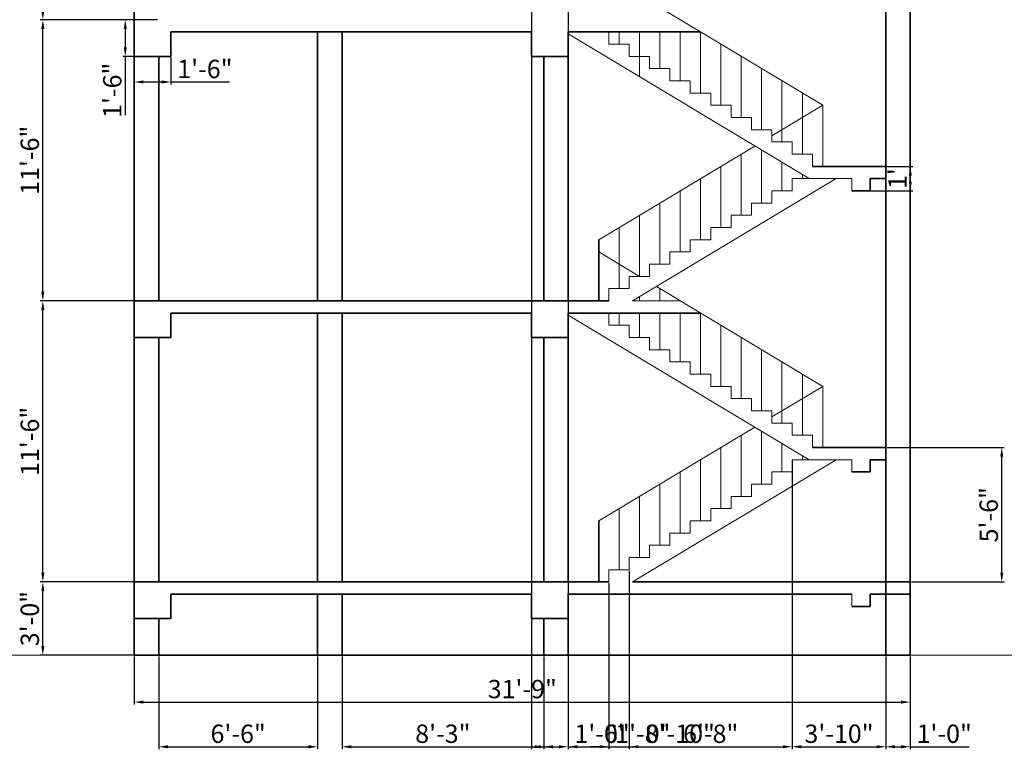
# Model space of a CAD drawing. Units: inches. Extents: x 1692 to 2762, y 798 to 1757.
# Tile 3 of 4: x 2279 to 2762, y 798 to 1156. Entities that reach past the tile are written whole.
import ezdxf

# ---------------------------------------------------------------- set-up
doc = ezdxf.new("R2010")
doc.units = ezdxf.units.IN
for name, color, linetype, lineweight in [('A-ANNO-DIMS', 2, 'Continuous', 18), ('A-CONS', 9, 'Continuous', 13), ('A-FLOR-STRS', 3, 'Continuous', 18), ('A-SECT', 1, 'Continuous', 35)]:
    doc.layers.add(name, color=color, linetype=linetype, lineweight=lineweight)
doc.styles.get("Standard").update_dxf_attribs({"font": 'arial.ttf'})
doc.dimstyles.new('ISO-25', dxfattribs={"dimtxt": 9, "dimasz": 4.5, "dimexe": 1.25, "dimexo": 0.625, "dimtad": 1, "dimdec": 0, "dimlunit": 3, "dimtxsty": 'Standard', "dimcen": 2.5, "dimadec": 0, "dimazin": 0, "dimtfac": 1, "dimtdec": 0, "dimtmove": 0, "dimatfit": 3, "dimfxl": 1, "dimarcsym": 0})

# ---------------------------------------------------------------- blocks, each defined once
blk = doc.blocks.new('*D4')
at = {"layer": 'A-ANNO-DIMS', "color": 0, "lineweight": -2, "transparency": 16777216}
for p, q in [((2334.78, 843.81), (2334.78, 820.21)), ((2715.78, 843.81), (2715.78, 820.21)), ((2339.28, 821.46), (2711.28, 821.46))]:
    blk.add_line(p, q, dxfattribs=at)
at = {"layer": 'A-ANNO-DIMS', "color": 0, "lineweight": 0, "transparency": 16777216}
for points in [[(2339.28, 822.21), (2339.28, 820.71), (2334.78, 821.46)], [(2711.28, 822.21), (2711.28, 820.71), (2715.78, 821.46)]]:
    blk.add_solid(points, dxfattribs=at)
at = {"layer": 'Defpoints', "color": 0, "lineweight": 0, "transparency": 16777216}
for p in [(2334.78, 844.43), (2715.78, 844.43), (2715.78, 821.46)]:
    blk.add_point(p, dxfattribs=at)
at = {"layer": 'A-ANNO-DIMS', "color": 0, "transparency": 16777216, "insert": (2525.28, 826.68), "char_height": 9, "attachment_point": 5}
blk.add_mtext('31\'-9"', dxfattribs=at)
blk = doc.blocks.new('*D5')
at = {"layer": 'A-ANNO-DIMS', "color": 0, "lineweight": -2, "transparency": 16777216}
for p, q in [((2346.16, 1156.43), (2329.11, 1156.43)), ((2330.36, 1151.93), (2330.36, 1142.93)), ((2346.16, 1138.43), (2329.11, 1138.43)), ((2330.36, 1138.43), (2330.36, 1109.61))]:
    blk.add_line(p, q, dxfattribs=at)
at = {"layer": 'A-ANNO-DIMS', "color": 0, "lineweight": 0, "transparency": 16777216}
for points in [[(2329.61, 1151.93), (2331.11, 1151.93), (2330.36, 1156.43)], [(2329.61, 1142.93), (2331.11, 1142.93), (2330.36, 1138.43)]]:
    blk.add_solid(points, dxfattribs=at)
at = {"layer": 'Defpoints', "color": 0, "lineweight": 0, "transparency": 16777216}
for p in [(2346.78, 1156.43), (2330.36, 1138.43), (2346.78, 1138.43)]:
    blk.add_point(p, dxfattribs=at)
at = {"layer": 'A-ANNO-DIMS', "color": 0, "transparency": 16777216, "insert": (2325.14, 1121.77), "char_height": 9, "attachment_point": 5, "rotation": 90}
blk.add_mtext('1\'-6"', dxfattribs=at)
blk = doc.blocks.new('*D6')
at = {"layer": 'A-ANNO-DIMS', "color": 0, "lineweight": -2, "transparency": 16777216}
for p, q in [((2334.78, 1137.81), (2334.78, 1124.62)), ((2352.78, 1137.81), (2352.78, 1124.62)), ((2339.28, 1125.87), (2348.28, 1125.87)), ((2352.78, 1125.87), (2381.61, 1125.87))]:
    blk.add_line(p, q, dxfattribs=at)
at = {"layer": 'A-ANNO-DIMS', "color": 0, "lineweight": 0, "transparency": 16777216}
for points in [[(2339.28, 1126.62), (2339.28, 1125.12), (2334.78, 1125.87)], [(2348.28, 1126.62), (2348.28, 1125.12), (2352.78, 1125.87)]]:
    blk.add_solid(points, dxfattribs=at)
at = {"layer": 'Defpoints', "color": 0, "lineweight": 0, "transparency": 16777216}
for p in [(2334.78, 1138.43), (2352.78, 1138.43), (2352.78, 1125.87)]:
    blk.add_point(p, dxfattribs=at)
at = {"layer": 'A-ANNO-DIMS', "color": 0, "transparency": 16777216, "insert": (2369.44, 1131.09), "char_height": 9, "attachment_point": 5}
blk.add_mtext('1\'-6"', dxfattribs=at)
blk = doc.blocks.new('*D11')
at = {"layer": 'A-ANNO-DIMS', "color": 0, "lineweight": -2, "transparency": 16777216}
for p, q in [((2687.74, 1084.43), (2717.03, 1084.43)), ((2715.78, 1076.93), (2715.78, 1079.93)), ((2687.74, 1072.43), (2717.03, 1072.43))]:
    blk.add_line(p, q, dxfattribs=at)
at = {"layer": 'A-ANNO-DIMS', "color": 0, "lineweight": 0, "transparency": 16777216}
for points in [[(2715.03, 1079.93), (2716.53, 1079.93), (2715.78, 1084.43)], [(2715.03, 1076.93), (2716.53, 1076.93), (2715.78, 1072.43)]]:
    blk.add_solid(points, dxfattribs=at)
at = {"layer": 'Defpoints', "color": 0, "lineweight": 0, "transparency": 16777216}
for p in [(2687.11, 1084.43), (2715.78, 1084.43), (2687.11, 1072.43)]:
    blk.add_point(p, dxfattribs=at)
at = {"layer": 'A-ANNO-DIMS', "color": 0, "transparency": 16777216, "insert": (2710.64, 1078.43), "char_height": 9, "attachment_point": 5, "rotation": 90}
blk.add_mtext("1'", dxfattribs=at)
blk = doc.blocks.new('*D51')
at = {"layer": 'A-ANNO-DIMS', "color": 0, "lineweight": -2, "transparency": 16777216}
for p, q in [((2334.16, 880.43), (2288.63, 880.43)), ((2289.88, 848.93), (2289.88, 875.93)), ((2334.16, 844.43), (2288.63, 844.43))]:
    blk.add_line(p, q, dxfattribs=at)
at = {"layer": 'A-ANNO-DIMS', "color": 0, "lineweight": 0, "transparency": 16777216}
for points in [[(2289.13, 875.93), (2290.63, 875.93), (2289.88, 880.43)], [(2289.13, 848.93), (2290.63, 848.93), (2289.88, 844.43)]]:
    blk.add_solid(points, dxfattribs=at)
at = {"layer": 'Defpoints', "color": 0, "lineweight": 0, "transparency": 16777216}
for p in [(2289.88, 880.43), (2334.78, 880.43), (2334.78, 844.43)]:
    blk.add_point(p, dxfattribs=at)
at = {"layer": 'A-ANNO-DIMS', "color": 0, "transparency": 16777216, "insert": (2284.66, 862.43), "char_height": 9, "attachment_point": 5, "rotation": 90}
blk.add_mtext('3\'-0"', dxfattribs=at)
blk = doc.blocks.new('*D52')
at = {"layer": 'A-ANNO-DIMS', "color": 0, "lineweight": -2, "transparency": 16777216}
for p, q in [((2334.16, 1018.43), (2288.63, 1018.43)), ((2289.88, 884.93), (2289.88, 1013.93)), ((2334.16, 880.43), (2288.63, 880.43))]:
    blk.add_line(p, q, dxfattribs=at)
at = {"layer": 'A-ANNO-DIMS', "color": 0, "lineweight": 0, "transparency": 16777216}
for points in [[(2289.13, 1013.93), (2290.63, 1013.93), (2289.88, 1018.43)], [(2289.13, 884.93), (2290.63, 884.93), (2289.88, 880.43)]]:
    blk.add_solid(points, dxfattribs=at)
at = {"layer": 'Defpoints', "color": 0, "lineweight": 0, "transparency": 16777216}
for p in [(2289.88, 1018.43), (2334.78, 1018.43), (2334.78, 880.43)]:
    blk.add_point(p, dxfattribs=at)
at = {"layer": 'A-ANNO-DIMS', "color": 0, "transparency": 16777216, "insert": (2284.66, 949.43), "char_height": 9, "attachment_point": 5, "rotation": 90}
blk.add_mtext('11\'-6"', dxfattribs=at)
blk = doc.blocks.new('*D53')
at = {"layer": 'A-ANNO-DIMS', "color": 0, "lineweight": -2, "transparency": 16777216}
for p, q in [((2334.16, 1156.43), (2288.63, 1156.43)), ((2289.88, 1022.93), (2289.88, 1151.93)), ((2334.16, 1018.43), (2288.63, 1018.43))]:
    blk.add_line(p, q, dxfattribs=at)
at = {"layer": 'A-ANNO-DIMS', "color": 0, "lineweight": 0, "transparency": 16777216}
for points in [[(2289.13, 1151.93), (2290.63, 1151.93), (2289.88, 1156.43)], [(2289.13, 1022.93), (2290.63, 1022.93), (2289.88, 1018.43)]]:
    blk.add_solid(points, dxfattribs=at)
at = {"layer": 'Defpoints', "color": 0, "lineweight": 0, "transparency": 16777216}
for p in [(2289.88, 1156.43), (2334.78, 1156.43), (2334.78, 1018.43)]:
    blk.add_point(p, dxfattribs=at)
at = {"layer": 'A-ANNO-DIMS', "color": 0, "transparency": 16777216, "insert": (2284.66, 1087.43), "char_height": 9, "attachment_point": 5, "rotation": 90}
blk.add_mtext('11\'-6"', dxfattribs=at)
blk = doc.blocks.new('*D54')
at = {"layer": 'A-ANNO-DIMS', "color": 0, "lineweight": -2, "transparency": 16777216}
for p, q in [((2334.16, 1294.43), (2288.63, 1294.43)), ((2289.88, 1160.93), (2289.88, 1289.93)), ((2334.16, 1156.43), (2288.63, 1156.43))]:
    blk.add_line(p, q, dxfattribs=at)
at = {"layer": 'A-ANNO-DIMS', "color": 0, "lineweight": 0, "transparency": 16777216}
for points in [[(2289.13, 1289.93), (2290.63, 1289.93), (2289.88, 1294.43)], [(2289.13, 1160.93), (2290.63, 1160.93), (2289.88, 1156.43)]]:
    blk.add_solid(points, dxfattribs=at)
at = {"layer": 'Defpoints', "color": 0, "lineweight": 0, "transparency": 16777216}
for p in [(2289.88, 1294.43), (2334.78, 1294.43), (2334.78, 1156.43)]:
    blk.add_point(p, dxfattribs=at)
at = {"layer": 'A-ANNO-DIMS', "color": 0, "transparency": 16777216, "insert": (2284.66, 1225.43), "char_height": 9, "attachment_point": 5, "rotation": 90}
blk.add_mtext('11\'-6"', dxfattribs=at)
blk = doc.blocks.new('*D57')
at = {"layer": 'A-ANNO-DIMS', "color": 0, "lineweight": -2, "transparency": 16777216}
for p, q in [((2346.78, 843.81), (2346.78, 798.28)), ((2424.78, 843.81), (2424.78, 798.28)), ((2351.28, 799.53), (2420.28, 799.53))]:
    blk.add_line(p, q, dxfattribs=at)
at = {"layer": 'A-ANNO-DIMS', "color": 0, "lineweight": 0, "transparency": 16777216}
for points in [[(2351.28, 800.28), (2351.28, 798.78), (2346.78, 799.53)], [(2420.28, 800.28), (2420.28, 798.78), (2424.78, 799.53)]]:
    blk.add_solid(points, dxfattribs=at)
at = {"layer": 'Defpoints', "color": 0, "lineweight": 0, "transparency": 16777216}
for p in [(2346.78, 844.43), (2424.78, 844.43), (2424.78, 799.53)]:
    blk.add_point(p, dxfattribs=at)
at = {"layer": 'A-ANNO-DIMS', "color": 0, "transparency": 16777216, "insert": (2385.78, 804.75), "char_height": 9, "attachment_point": 5}
blk.add_mtext('6\'-6"', dxfattribs=at)
blk = doc.blocks.new('*D58')
at = {"layer": 'A-ANNO-DIMS', "color": 0, "lineweight": -2, "transparency": 16777216}
for p, q in [((2436.78, 843.81), (2436.78, 798.28)), ((2535.78, 843.81), (2535.78, 798.28)), ((2441.28, 799.53), (2531.28, 799.53))]:
    blk.add_line(p, q, dxfattribs=at)
at = {"layer": 'A-ANNO-DIMS', "color": 0, "lineweight": 0, "transparency": 16777216}
for points in [[(2441.28, 800.28), (2441.28, 798.78), (2436.78, 799.53)], [(2531.28, 800.28), (2531.28, 798.78), (2535.78, 799.53)]]:
    blk.add_solid(points, dxfattribs=at)
at = {"layer": 'Defpoints', "color": 0, "lineweight": 0, "transparency": 16777216}
for p in [(2436.78, 844.43), (2535.78, 844.43), (2535.78, 799.53)]:
    blk.add_point(p, dxfattribs=at)
at = {"layer": 'A-ANNO-DIMS', "color": 0, "transparency": 16777216, "insert": (2486.28, 804.76), "char_height": 9, "attachment_point": 5}
blk.add_mtext('8\'-3"', dxfattribs=at)
blk = doc.blocks.new('*D59')
at = {"layer": 'A-ANNO-DIMS', "color": 0, "lineweight": -2, "transparency": 16777216}
for p, q in [((2535.78, 843.81), (2535.78, 798.28)), ((2547.78, 843.81), (2547.78, 798.28)), ((2540.28, 799.53), (2543.28, 799.53)), ((2547.78, 799.53), (2576.61, 799.53))]:
    blk.add_line(p, q, dxfattribs=at)
at = {"layer": 'A-ANNO-DIMS', "color": 0, "lineweight": 0, "transparency": 16777216}
for points in [[(2540.28, 800.28), (2540.28, 798.78), (2535.78, 799.53)], [(2543.28, 800.28), (2543.28, 798.78), (2547.78, 799.53)]]:
    blk.add_solid(points, dxfattribs=at)
at = {"layer": 'Defpoints', "color": 0, "lineweight": 0, "transparency": 16777216}
for p in [(2535.78, 844.43), (2547.78, 844.43), (2547.78, 799.53)]:
    blk.add_point(p, dxfattribs=at)
at = {"layer": 'A-ANNO-DIMS', "color": 0, "transparency": 16777216, "insert": (2564.44, 804.75), "char_height": 9, "attachment_point": 5}
blk.add_mtext('1\'-0"', dxfattribs=at)
blk = doc.blocks.new('*D60')
at = {"layer": 'A-ANNO-DIMS', "color": 0, "lineweight": -2, "transparency": 16777216}
for p, q in [((2567.78, 879.81), (2567.78, 798.28)), ((2547.78, 843.81), (2547.78, 798.28)), ((2552.28, 799.53), (2563.28, 799.53)), ((2567.78, 799.53), (2596.61, 799.53))]:
    blk.add_line(p, q, dxfattribs=at)
at = {"layer": 'A-ANNO-DIMS', "color": 0, "lineweight": 0, "transparency": 16777216}
for points in [[(2552.28, 800.28), (2552.28, 798.78), (2547.78, 799.53)], [(2563.28, 800.28), (2563.28, 798.78), (2567.78, 799.53)]]:
    blk.add_solid(points, dxfattribs=at)
at = {"layer": 'Defpoints', "color": 0, "lineweight": 0, "transparency": 16777216}
for p in [(2567.78, 880.43), (2547.78, 844.43), (2567.78, 799.53)]:
    blk.add_point(p, dxfattribs=at)
at = {"layer": 'A-ANNO-DIMS', "color": 0, "transparency": 16777216, "insert": (2584.44, 804.75), "char_height": 9, "attachment_point": 5}
blk.add_mtext('1\'-8"', dxfattribs=at)
blk = doc.blocks.new('*D61')
at = {"layer": 'A-ANNO-DIMS', "color": 0, "lineweight": -2, "transparency": 16777216}
for p, q in [((2577.78, 885.81), (2577.78, 798.28)), ((2567.78, 879.81), (2567.78, 798.28)), ((2563.28, 799.53), (2558.78, 799.53)), ((2567.78, 799.53), (2577.78, 799.53)), ((2582.28, 799.53), (2618.95, 799.53))]:
    blk.add_line(p, q, dxfattribs=at)
at = {"layer": 'A-ANNO-DIMS', "color": 0, "lineweight": 0, "transparency": 16777216}
for points in [[(2563.28, 800.28), (2563.28, 798.78), (2567.78, 799.53)], [(2582.28, 800.28), (2582.28, 798.78), (2577.78, 799.53)]]:
    blk.add_solid(points, dxfattribs=at)
at = {"layer": 'Defpoints', "color": 0, "lineweight": 0, "transparency": 16777216}
for p in [(2577.78, 886.43), (2567.78, 880.43), (2577.78, 799.53)]:
    blk.add_point(p, dxfattribs=at)
at = {"layer": 'A-ANNO-DIMS', "color": 0, "transparency": 16777216, "insert": (2602.86, 804.75), "char_height": 9, "attachment_point": 5}
blk.add_mtext('0\'-10"', dxfattribs=at)
blk = doc.blocks.new('*D62')
at = {"layer": 'A-ANNO-DIMS', "color": 0, "lineweight": -2, "transparency": 16777216}
for p, q in [((2657.78, 939.81), (2657.78, 798.28)), ((2577.78, 885.81), (2577.78, 798.28)), ((2582.28, 799.53), (2653.28, 799.53))]:
    blk.add_line(p, q, dxfattribs=at)
at = {"layer": 'A-ANNO-DIMS', "color": 0, "lineweight": 0, "transparency": 16777216}
for points in [[(2582.28, 800.28), (2582.28, 798.78), (2577.78, 799.53)], [(2653.28, 800.28), (2653.28, 798.78), (2657.78, 799.53)]]:
    blk.add_solid(points, dxfattribs=at)
at = {"layer": 'Defpoints', "color": 0, "lineweight": 0, "transparency": 16777216}
for p in [(2657.78, 940.43), (2577.78, 886.43), (2657.78, 799.53)]:
    blk.add_point(p, dxfattribs=at)
at = {"layer": 'A-ANNO-DIMS', "color": 0, "transparency": 16777216, "insert": (2617.78, 804.75), "char_height": 9, "attachment_point": 5}
blk.add_mtext('6\'-8"', dxfattribs=at)
blk = doc.blocks.new('*D63')
at = {"layer": 'A-ANNO-DIMS', "color": 0, "lineweight": -2, "transparency": 16777216}
for p, q in [((2657.78, 939.81), (2657.78, 798.28)), ((2703.78, 843.81), (2703.78, 798.28)), ((2662.28, 799.53), (2699.28, 799.53))]:
    blk.add_line(p, q, dxfattribs=at)
at = {"layer": 'A-ANNO-DIMS', "color": 0, "lineweight": 0, "transparency": 16777216}
for points in [[(2662.28, 800.28), (2662.28, 798.78), (2657.78, 799.53)], [(2699.28, 800.28), (2699.28, 798.78), (2703.78, 799.53)]]:
    blk.add_solid(points, dxfattribs=at)
at = {"layer": 'Defpoints', "color": 0, "lineweight": 0, "transparency": 16777216}
for p in [(2657.78, 940.43), (2703.78, 844.43), (2703.78, 799.53)]:
    blk.add_point(p, dxfattribs=at)
at = {"layer": 'A-ANNO-DIMS', "color": 0, "transparency": 16777216, "insert": (2680.78, 804.76), "char_height": 9, "attachment_point": 5}
blk.add_mtext('3\'-10"', dxfattribs=at)
blk = doc.blocks.new('*D64')
at = {"layer": 'A-ANNO-DIMS', "color": 0, "lineweight": -2, "transparency": 16777216}
for p, q in [((2703.78, 843.81), (2703.78, 798.28)), ((2715.78, 843.81), (2715.78, 798.28)), ((2708.28, 799.53), (2711.28, 799.53)), ((2715.78, 799.53), (2744.61, 799.53))]:
    blk.add_line(p, q, dxfattribs=at)
at = {"layer": 'A-ANNO-DIMS', "color": 0, "lineweight": 0, "transparency": 16777216}
for points in [[(2708.28, 800.28), (2708.28, 798.78), (2703.78, 799.53)], [(2711.28, 800.28), (2711.28, 798.78), (2715.78, 799.53)]]:
    blk.add_solid(points, dxfattribs=at)
at = {"layer": 'Defpoints', "color": 0, "lineweight": 0, "transparency": 16777216}
for p in [(2703.78, 844.43), (2715.78, 844.43), (2715.78, 799.53)]:
    blk.add_point(p, dxfattribs=at)
at = {"layer": 'A-ANNO-DIMS', "color": 0, "transparency": 16777216, "insert": (2732.44, 804.75), "char_height": 9, "attachment_point": 5}
blk.add_mtext('1\'-0"', dxfattribs=at)
blk = doc.blocks.new('*D65')
at = {"layer": 'A-ANNO-DIMS', "color": 0, "lineweight": -2, "transparency": 16777216}
for p, q in [((2529.78, 1551.81), (2529.78, 798.28)), ((2547.78, 1551.81), (2547.78, 798.28)), ((2534.28, 799.53), (2543.28, 799.53)), ((2547.78, 799.53), (2576.61, 799.53))]:
    blk.add_line(p, q, dxfattribs=at)
at = {"layer": 'A-ANNO-DIMS', "color": 0, "lineweight": 0, "transparency": 16777216}
for points in [[(2534.28, 800.28), (2534.28, 798.78), (2529.78, 799.53)], [(2543.28, 800.28), (2543.28, 798.78), (2547.78, 799.53)]]:
    blk.add_solid(points, dxfattribs=at)
at = {"layer": 'Defpoints', "color": 0, "lineweight": 0, "transparency": 16777216}
for p in [(2529.78, 1552.43), (2547.78, 1552.43), (2547.78, 799.53)]:
    blk.add_point(p, dxfattribs=at)
at = {"layer": 'A-ANNO-DIMS', "color": 0, "transparency": 16777216, "insert": (2564.44, 804.75), "char_height": 9, "attachment_point": 5}
blk.add_mtext('1\'-6"', dxfattribs=at)
blk = doc.blocks.new('*D66')
at = {"layer": 'A-ANNO-DIMS', "color": 0, "lineweight": -2, "transparency": 16777216}
for p, q in [((2704.41, 946.43), (2761.93, 946.43)), ((2760.68, 884.93), (2760.68, 941.93)), ((2716.41, 880.43), (2761.93, 880.43))]:
    blk.add_line(p, q, dxfattribs=at)
at = {"layer": 'A-ANNO-DIMS', "color": 0, "lineweight": 0, "transparency": 16777216}
for points in [[(2759.93, 941.93), (2761.43, 941.93), (2760.68, 946.43)], [(2759.93, 884.93), (2761.43, 884.93), (2760.68, 880.43)]]:
    blk.add_solid(points, dxfattribs=at)
at = {"layer": 'Defpoints', "color": 0, "lineweight": 0, "transparency": 16777216}
for p in [(2703.78, 946.43), (2760.68, 946.43), (2715.78, 880.43)]:
    blk.add_point(p, dxfattribs=at)
at = {"layer": 'A-ANNO-DIMS', "color": 0, "transparency": 16777216, "insert": (2755.46, 913.43), "char_height": 9, "attachment_point": 5, "rotation": 90}
blk.add_mtext('5\'-6"', dxfattribs=at)

msp = doc.modelspace()

# ---------------------------------------------------------------- linework, layer by layer
at = {"layer": 'A-CONS'}
msp.add_xline((2166.78, 844.43), (1, 0), dxfattribs=at)
at = {"layer": 'A-FLOR-STRS'}
for p, q in [((2591.11, 1163.43), (2672.78, 1114.43)), ((2547.78, 1149.44), (2666.12, 1078.43)), ((2567.78, 1144.43), (2567.78, 1150.43)), ((2572.78, 1144.43), (2572.78, 1150.43)), ((2582.78, 1128.44), (2582.78, 1150.43)), ((2592.78, 1132.43), (2592.78, 1150.43)), ((2602.78, 1126.43), (2602.78, 1150.43)), ((2612.78, 1120.43), (2612.78, 1150.43)), ((2577.78, 1144.43), (2567.78, 1144.43)), ((2577.78, 1138.43), (2577.78, 1144.43)), ((2622.78, 1114.43), (2622.78, 1144.43)), ((2587.78, 1138.43), (2577.78, 1138.43)), ((2587.78, 1132.43), (2587.78, 1138.43)), ((2632.78, 1108.43), (2632.78, 1138.43)), ((2597.78, 1132.43), (2587.78, 1132.43)), ((2597.78, 1126.43), (2597.78, 1132.43)), ((2642.78, 1102.43), (2642.78, 1132.43)), ((2607.78, 1126.43), (2597.78, 1126.43)), ((2607.78, 1120.43), (2607.78, 1126.43)), ((2652.78, 1096.43), (2652.78, 1126.43)), ((2617.78, 1120.43), (2607.78, 1120.43)), ((2617.78, 1114.43), (2617.78, 1120.43)), ((2662.78, 1090.43), (2662.78, 1120.43)), ((2627.78, 1114.43), (2617.78, 1114.43)), ((2627.78, 1108.43), (2627.78, 1114.43)), ((2672.78, 1114.43), (2647.78, 1099.43)), ((2672.78, 1084.43), (2672.78, 1114.43)), ((2672.78, 1090.43), (2672.78, 1114.43)), ((2637.78, 1108.43), (2627.78, 1108.43)), ((2637.78, 1102.43), (2637.78, 1108.43)), ((2662.78, 1090.43), (2662.78, 1108.43)), ((2647.78, 1102.43), (2637.78, 1102.43)), ((2647.78, 1096.43), (2647.78, 1102.43)), ((2652.78, 1096.43), (2652.78, 1102.43)), ((2639.45, 1094.43), (2562.78, 1048.43)), ((2657.78, 1096.43), (2647.78, 1096.43)), ((2657.78, 1090.43), (2657.78, 1096.43)), ((2632.78, 1060.43), (2632.78, 1090.43)), ((2642.78, 1066.43), (2642.78, 1092.44)), ((2667.78, 1090.43), (2657.78, 1090.43)), ((2667.78, 1084.43), (2667.78, 1090.43)), ((2672.78, 1084.43), (2672.78, 1090.43)), ((2622.78, 1054.43), (2622.78, 1084.43)), ((2652.78, 1072.43), (2652.78, 1086.44)), ((2579.44, 1018.43), (2679.44, 1078.43)), ((2612.78, 1048.43), (2612.78, 1078.43)), ((2657.78, 1072.43), (2657.78, 1078.43)), ((2657.78, 1078.43), (2667.78, 1078.43)), ((2662.78, 1078.43), (2662.78, 1080.44)), ((2667.78, 1078.43), (2687.11, 1078.43)), ((2687.11, 1078.43), (2687.11, 1072.43)), ((2602.78, 1042.43), (2602.78, 1072.43)), ((2647.78, 1066.43), (2647.78, 1072.43)), ((2647.78, 1072.43), (2657.78, 1072.43)), ((2592.78, 1036.43), (2592.78, 1066.43)), ((2637.78, 1060.43), (2637.78, 1066.43)), ((2637.78, 1066.43), (2647.78, 1066.43)), ((2582.78, 1030.43), (2582.78, 1060.43)), ((2627.78, 1054.43), (2627.78, 1060.43)), ((2627.78, 1060.43), (2637.78, 1060.43)), ((2572.78, 1024.43), (2572.78, 1054.43)), ((2617.78, 1048.43), (2617.78, 1054.43)), ((2617.78, 1054.43), (2627.78, 1054.43)), ((2607.78, 1042.43), (2607.78, 1048.43)), ((2607.78, 1048.43), (2617.78, 1048.43)), ((2562.78, 1042.43), (2582.78, 1030.43)), ((2597.78, 1036.43), (2597.78, 1042.43)), ((2597.78, 1042.43), (2607.78, 1042.43)), ((2572.78, 1024.43), (2572.78, 1036.43)), ((2587.78, 1030.43), (2587.78, 1036.43)), ((2587.78, 1036.43), (2597.78, 1036.43)), ((2577.78, 1024.43), (2577.78, 1030.43)), ((2577.78, 1030.43), (2587.78, 1030.43)), ((2591.11, 1025.43), (2672.78, 976.43)), ((2567.78, 1018.43), (2567.78, 1024.43)), ((2567.78, 1024.43), (2577.78, 1024.43)), ((2582.78, 1018.43), (2582.78, 1020.44)), ((2592.78, 1018.43), (2592.78, 1024.43)), ((2579.44, 1018.43), (2602.78, 1018.43)), ((2547.78, 1011.44), (2666.12, 940.43)), ((2567.78, 1012.43), (2567.78, 1006.43)), ((2572.78, 1006.43), (2572.78, 1012.43)), ((2582.78, 1000.43), (2582.78, 1012.43)), ((2592.78, 994.43), (2592.78, 1012.43)), ((2602.78, 988.43), (2602.78, 1012.43)), ((2612.78, 982.43), (2612.78, 1012.43)), ((2577.78, 1006.43), (2567.78, 1006.43)), ((2577.78, 1000.43), (2577.78, 1006.43)), ((2622.78, 976.43), (2622.78, 1006.43)), ((2587.78, 1000.43), (2577.78, 1000.43)), ((2587.78, 994.43), (2587.78, 1000.43)), ((2632.78, 970.43), (2632.78, 1000.43)), ((2597.78, 994.43), (2587.78, 994.43)), ((2597.78, 988.43), (2597.78, 994.43)), ((2642.78, 964.43), (2642.78, 994.43)), ((2607.78, 988.43), (2597.78, 988.43)), ((2607.78, 982.43), (2607.78, 988.43)), ((2652.78, 958.43), (2652.78, 988.43)), ((2617.78, 982.43), (2607.78, 982.43)), ((2617.78, 976.43), (2617.78, 982.43)), ((2662.78, 952.43), (2662.78, 982.43)), ((2627.78, 976.43), (2617.78, 976.43)), ((2627.78, 970.43), (2627.78, 976.43)), ((2672.78, 976.43), (2647.78, 961.43)), ((2672.78, 946.43), (2672.78, 976.43)), ((2672.78, 952.43), (2672.78, 976.43)), ((2637.78, 970.43), (2627.78, 970.43)), ((2637.78, 964.43), (2637.78, 970.43)), ((2662.78, 952.43), (2662.78, 970.43)), ((2647.78, 964.43), (2637.78, 964.43)), ((2647.78, 958.43), (2647.78, 964.43)), ((2652.78, 958.43), (2652.78, 964.43)), ((2657.78, 958.43), (2647.78, 958.43)), ((2657.78, 952.43), (2657.78, 958.43)), ((2639.45, 956.43), (2562.78, 910.43)), ((2632.78, 922.43), (2632.78, 952.43)), ((2642.78, 928.43), (2642.78, 954.44)), ((2667.78, 952.43), (2657.78, 952.43)), ((2667.78, 946.43), (2667.78, 952.43)), ((2672.78, 946.43), (2672.78, 952.43)), ((2652.78, 934.43), (2652.78, 948.44)), ((2622.78, 916.43), (2622.78, 946.43)), ((2579.44, 880.43), (2679.44, 940.43)), ((2612.78, 910.43), (2612.78, 940.43)), ((2657.78, 934.43), (2657.78, 940.43)), ((2657.78, 940.43), (2667.78, 940.43)), ((2662.78, 940.43), (2662.78, 942.44)), ((2667.78, 940.43), (2687.11, 940.43)), ((2687.11, 940.43), (2687.11, 934.43)), ((2602.78, 904.43), (2602.78, 934.43)), ((2647.78, 928.43), (2647.78, 934.43)), ((2647.78, 934.43), (2657.78, 934.43)), ((2592.78, 898.43), (2592.78, 928.43)), ((2637.78, 922.43), (2637.78, 928.43)), ((2637.78, 928.43), (2647.78, 928.43)), ((2582.78, 892.43), (2582.78, 922.43)), ((2627.78, 916.43), (2627.78, 922.43)), ((2627.78, 922.43), (2637.78, 922.43)), ((2572.78, 886.43), (2572.78, 916.43)), ((2617.78, 910.43), (2617.78, 916.43)), ((2617.78, 916.43), (2627.78, 916.43)), ((2607.78, 904.43), (2607.78, 910.43)), ((2607.78, 910.43), (2617.78, 910.43)), ((2597.78, 898.43), (2597.78, 904.43)), ((2597.78, 904.43), (2607.78, 904.43)), ((2587.78, 892.43), (2587.78, 898.43)), ((2587.78, 898.43), (2597.78, 898.43)), ((2577.78, 886.43), (2577.78, 892.43)), ((2577.78, 892.43), (2587.78, 892.43)), ((2567.78, 880.43), (2567.78, 886.43)), ((2567.78, 886.43), (2577.78, 886.43)), ((2687.11, 874.43), (2687.11, 868.43))]:
    msp.add_line(p, q, dxfattribs=at)
at = {"layer": 'A-SECT'}
for p, q in [((2715.78, 1708.43), (2715.78, 844.43)), ((2703.78, 1678.43), (2703.78, 844.43)), ((2334.78, 1612.43), (2334.78, 844.43)), ((2352.78, 1150.43), (2529.78, 1150.43)), ((2352.78, 1150.43), (2352.78, 1138.43)), ((2424.78, 1150.43), (2424.78, 1018.43)), ((2436.78, 1150.43), (2436.78, 1018.43)), ((2529.78, 1150.43), (2529.78, 1138.43)), ((2547.78, 1150.43), (2612.78, 1150.43)), ((2547.78, 1150.43), (2547.78, 1018.43)), ((2334.78, 1138.43), (2352.78, 1138.43)), ((2346.78, 1138.43), (2346.78, 1018.43)), ((2529.78, 1138.43), (2547.78, 1138.43)), ((2535.78, 1138.43), (2535.78, 1018.43)), ((2667.78, 1084.43), (2703.78, 1084.43)), ((2696.11, 1078.43), (2696.11, 1072.43)), ((2696.11, 1078.43), (2703.78, 1078.43)), ((2687.11, 1072.43), (2696.11, 1072.43)), ((2562.78, 1018.43), (2562.78, 1048.43)), ((2562.78, 1018.43), (2562.78, 1042.43)), ((2334.78, 1018.43), (2567.78, 1018.43)), ((2352.78, 1012.43), (2352.78, 1000.43)), ((2352.78, 1012.43), (2529.78, 1012.43)), ((2424.78, 1012.43), (2424.78, 880.43)), ((2436.78, 1012.43), (2436.78, 880.43)), ((2529.78, 1012.43), (2529.78, 1000.43)), ((2547.78, 1012.43), (2612.78, 1012.43)), ((2547.78, 1012.43), (2547.78, 880.43)), ((2334.78, 1000.43), (2352.78, 1000.43)), ((2346.78, 1000.43), (2346.78, 880.43)), ((2529.78, 1000.43), (2547.78, 1000.43)), ((2535.78, 1000.43), (2535.78, 880.43)), ((2667.78, 946.43), (2703.78, 946.43)), ((2696.11, 940.43), (2696.11, 934.43)), ((2696.11, 940.43), (2703.78, 940.43)), ((2687.11, 934.43), (2696.11, 934.43)), ((2562.78, 880.43), (2562.78, 910.43)), ((2562.78, 880.43), (2562.78, 886.43)), ((2334.78, 880.43), (2567.78, 880.43)), ((2579.44, 880.43), (2715.78, 880.43)), ((2352.78, 874.43), (2529.78, 874.43)), ((2352.78, 874.43), (2352.78, 862.43)), ((2424.78, 874.43), (2424.78, 844.43)), ((2436.78, 874.43), (2436.78, 844.43)), ((2529.78, 874.43), (2529.78, 862.43)), ((2547.78, 874.43), (2687.11, 874.43)), ((2547.78, 874.43), (2547.78, 844.43)), ((2696.11, 874.43), (2696.11, 868.43)), ((2696.11, 874.43), (2715.78, 874.43)), ((2687.11, 868.43), (2696.11, 868.43)), ((2334.78, 862.43), (2352.78, 862.43)), ((2346.78, 862.43), (2346.78, 844.43)), ((2529.78, 862.43), (2547.78, 862.43)), ((2535.78, 862.43), (2535.78, 844.43)), ((2334.78, 844.43), (2715.78, 844.43))]:
    msp.add_line(p, q, dxfattribs=at)

# ---------------------------------------------------------------- dimensions: what is measured, and where the dimension line sits
at = {"layer": 'A-ANNO-DIMS'}
for base, p1, p2, override, picture, middle in [((2547.78, 799.53), (2529.78, 1552.43), (2547.78, 1552.43), {"dimdec": 1, "dimlfac": 1, "dimrnd": 0, "dimzin": 1, "dimdsep": 46, "dimlunit": 4, "dimfrac": 2}, '*D65', (2564.44, 804.75)), ((2352.78, 1125.87), (2334.78, 1138.43), (2352.78, 1138.43), {"dimclrd": 0, "dimclre": 0, "dimclrt": 0}, '*D6', (2369.44, 1131.09)), ((2657.78, 799.53), (2577.78, 886.43), (2657.78, 940.43), {"dimdec": 1, "dimlfac": 1, "dimrnd": 0, "dimzin": 1, "dimdsep": 46, "dimlunit": 4, "dimfrac": 2}, '*D62', (2617.78, 804.75)), ((2703.78, 799.53), (2657.78, 940.43), (2703.78, 844.43), {"dimdec": 1, "dimlfac": 1, "dimrnd": 0, "dimzin": 1, "dimdsep": 46, "dimlunit": 4, "dimfrac": 2}, '*D63', (2680.78, 804.76)), ((2577.78, 799.53), (2567.78, 880.43), (2577.78, 886.43), {"dimdec": 1, "dimlfac": 1, "dimrnd": 0, "dimzin": 1, "dimdsep": 46, "dimlunit": 4, "dimfrac": 2}, '*D61', (2602.86, 804.75)), ((2567.78, 799.53), (2547.78, 844.43), (2567.78, 880.43), {"dimdec": 1, "dimlfac": 1, "dimrnd": 0, "dimzin": 1, "dimdsep": 46, "dimlunit": 4, "dimfrac": 2}, '*D60', (2584.44, 804.75)), ((2715.78, 821.46), (2334.78, 844.43), (2715.78, 844.43), {"dimclrd": 0, "dimclre": 0, "dimclrt": 0}, '*D4', (2525.28, 826.68)), ((2424.78, 799.53), (2346.78, 844.43), (2424.78, 844.43), {"dimdec": 1, "dimlfac": 1, "dimrnd": 0, "dimzin": 1, "dimdsep": 46, "dimlunit": 4, "dimfrac": 2}, '*D57', (2385.78, 804.75)), ((2535.78, 799.53), (2436.78, 844.43), (2535.78, 844.43), {"dimdec": 1, "dimlfac": 1, "dimrnd": 0, "dimzin": 1, "dimdsep": 46, "dimlunit": 4, "dimfrac": 2}, '*D58', (2486.28, 804.76)), ((2547.78, 799.53), (2535.78, 844.43), (2547.78, 844.43), {"dimdec": 1, "dimlfac": 1, "dimrnd": 0, "dimzin": 1, "dimdsep": 46, "dimlunit": 4, "dimfrac": 2}, '*D59', (2564.44, 804.75)), ((2715.78, 799.53), (2703.78, 844.43), (2715.78, 844.43), {"dimdec": 1, "dimlfac": 1, "dimrnd": 0, "dimzin": 1, "dimdsep": 46, "dimlunit": 4, "dimfrac": 2}, '*D64', (2732.44, 804.75))]:
    dim = msp.add_linear_dim(base=base, p1=p1, p2=p2, dimstyle='ISO-25', override=override, dxfattribs=at)
    dim.commit()
    dim.dimension.update_dxf_attribs({"geometry": picture, "text_midpoint": middle})
for base, p1, p2, override, picture, middle in [((2289.88, 1294.43), (2334.78, 1156.43), (2334.78, 1294.43), {"dimdec": 1, "dimlfac": 1, "dimrnd": 0, "dimzin": 1, "dimdsep": 46, "dimlunit": 4, "dimfrac": 2}, '*D54', (2284.66, 1225.43)), ((2289.88, 1156.43), (2334.78, 1018.43), (2334.78, 1156.43), {"dimdec": 1, "dimlfac": 1, "dimrnd": 0, "dimzin": 1, "dimdsep": 46, "dimlunit": 4, "dimfrac": 2}, '*D53', (2284.66, 1087.43)), ((2330.36, 1138.43), (2346.78, 1156.43), (2346.78, 1138.43), {"dimclrd": 0, "dimclre": 0, "dimclrt": 0}, '*D5', (2325.14, 1121.77)), ((2715.78, 1084.43), (2687.11, 1072.43), (2687.11, 1084.43), {"dimclrd": 0, "dimclre": 0, "dimclrt": 0}, '*D11', (2710.64, 1078.43)), ((2289.88, 1018.43), (2334.78, 880.43), (2334.78, 1018.43), {"dimdec": 1, "dimlfac": 1, "dimrnd": 0, "dimzin": 1, "dimdsep": 46, "dimlunit": 4, "dimfrac": 2}, '*D52', (2284.66, 949.43)), ((2760.68, 946.43), (2715.78, 880.43), (2703.78, 946.43), {"dimdec": 1, "dimlfac": 1, "dimrnd": 0, "dimzin": 1, "dimdsep": 46, "dimlunit": 4, "dimfrac": 2}, '*D66', (2755.46, 913.43)), ((2289.88, 880.43), (2334.78, 844.43), (2334.78, 880.43), {"dimdec": 1, "dimlfac": 1, "dimrnd": 0, "dimzin": 1, "dimdsep": 46, "dimlunit": 4, "dimfrac": 2}, '*D51', (2284.66, 862.43))]:
    dim = msp.add_linear_dim(base=base, p1=p1, p2=p2, angle=90, dimstyle='ISO-25', override=override, dxfattribs=at)
    dim.commit()
    dim.dimension.update_dxf_attribs({"geometry": picture, "text_midpoint": middle})

doc.saveas('drawing.dxf')
